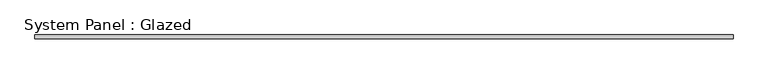
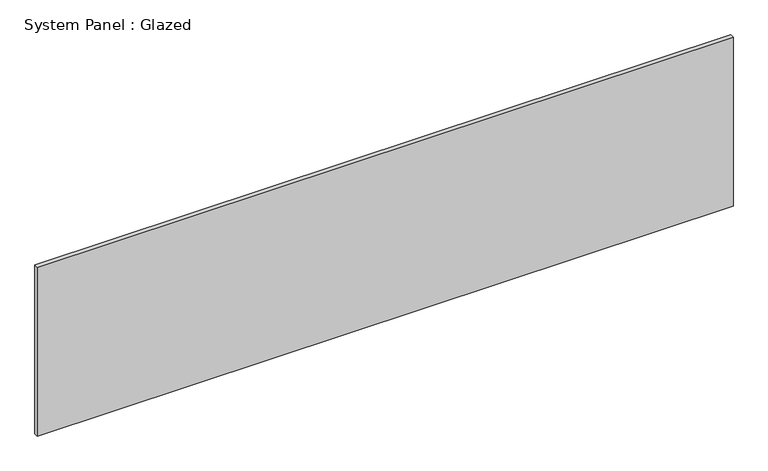
"""IFC4 building model written with IfcOpenShell, lengths in millimetres: plate geometry, System Panel : Glazed."""

from ifc_helpers import new_model, si_unit, origin, origin_with_axes, place, context, project, spatial, polyline, outline, extrude, source, transform, mapped, element, save


def system_panel_glazed_2a610dff(model_context):
    return source(origin(), model_context, "Body", "SweptSolid", [
        extrude(outline(polyline([(2251.3569113, 19.05), (-2251.3569113, 19.05), (-2251.3569113, 44.45), (2251.3569113, 44.45), (2251.3569113, 19.05)])), origin_with_axes(), (0.0, 0.0, 1.0), 1155.7),
    ])


if __name__ == "__main__":
    model = new_model("IFC4")
    model_context = context("Model", 3, world=origin())
    ifc_project = project(units=[si_unit("LENGTHUNIT", "METRE", prefix="MILLI")], contexts=[model_context])
    site = spatial("IfcSite", under=ifc_project)
    building = spatial("IfcBuilding", under=site)
    placement = place(None, origin())
    system_panel_glazed_shape = system_panel_glazed_2a610dff(model_context)
    element("IfcPlate", 1, ObjectType="System Panel : Glazed", at=placement, inside=building, context=model_context, shape_type="MappedRepresentation", body=[
        mapped(system_panel_glazed_shape, transform((0.0, 0.0, 0.0), x_axis=(1.0, 0.0, 0.0), y_axis=(0.0, 1.0, 0.0), z_axis=(0.0, 0.0, 1.0))),
    ])
    save(model, "model.ifc")

# Revit data of these elements
# Type "System Panel : Glazed"
#   Construction Type Id = "GSP4R"
#   Analytic Construction = "1/8 in Pilkington single glazing"
#   Visual Light Transmittance = 0.9
#   Solar Heat Gain Coefficient = 0.86
#   Heat Transfer Coefficient (U) = 1.18115 BTU/(h·ft²·°F)
# Element 1 (IfcPlate, "System Panel : Glazed")
#   Materials on its faces: "Glass"
# Materials
#   "Glass": class "Glass", colour RGB 0 128 192, transparency 0.75, Description = "Soda Lime Glass", Cost = 0
